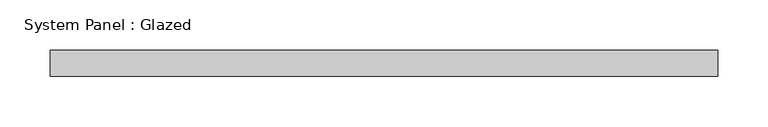
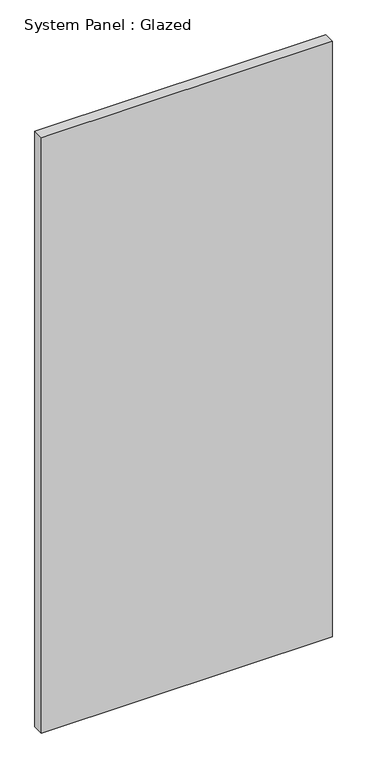
"""IFC4 building model written with IfcOpenShell, lengths in millimetres: plate geometry, System Panel : Glazed."""

from ifc_helpers import new_model, si_unit, origin, origin_with_axes, place, context, project, spatial, polyline, outline, extrude, source, transform, mapped, element, save


def system_panel_glazed_33375d59(model_context):
    return source(origin(), model_context, "Body", "SweptSolid", [
        extrude(outline(polyline([(330.2, 19.05), (-330.2, 19.05), (-330.2, 44.45), (330.2, 44.45), (330.2, 19.05)])), origin_with_axes(), (0.0, 0.0, 1.0), 1430.357611),
    ])


if __name__ == "__main__":
    model = new_model("IFC4")
    model_context = context("Model", 3, world=origin())
    ifc_project = project(units=[si_unit("LENGTHUNIT", "METRE", prefix="MILLI")], contexts=[model_context])
    site = spatial("IfcSite", under=ifc_project)
    building = spatial("IfcBuilding", under=site)
    placement = place(None, origin())
    system_panel_glazed_shape = system_panel_glazed_33375d59(model_context)
    element("IfcPlate", 1, ObjectType="System Panel : Glazed", at=placement, inside=building, context=model_context, shape_type="MappedRepresentation", body=[
        mapped(system_panel_glazed_shape, transform((0.0, 0.0, 0.0), x_axis=(1.0, 0.0, 0.0), y_axis=(0.0, 1.0, 0.0), z_axis=(0.0, 0.0, 1.0))),
    ])
    save(model, "model.ifc")

# Revit data of these elements
# Type "System Panel : Glazed"
#   Construction Type Id = "GSP4R"
#   Analytic Construction = "1/8 in Pilkington single glazing"
#   Visual Light Transmittance = 0.9
#   Solar Heat Gain Coefficient = 0.86
#   Heat Transfer Coefficient (U) = 1.18115 BTU/(h·ft²·°F)
#   Define Thermal Properties by = 1
# Element 1 (IfcPlate, "System Panel : Glazed")
#   Materials on its faces: "Glass"
# Materials
#   "Glass": class "Glass", colour RGB 0 128 192, transparency 0.75, Description = "Soda Lime Glass", Cost = 0
